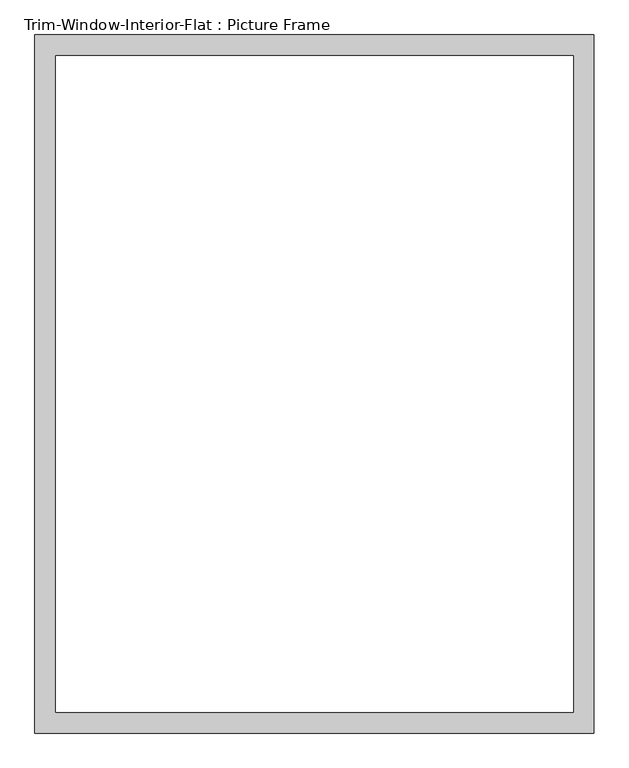
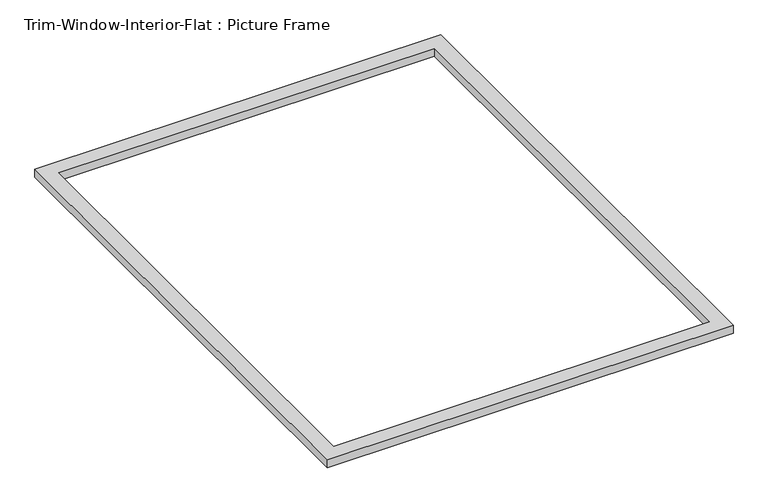
"""IFC4 building model written with IfcOpenShell, lengths in millimetres: proxy geometry, Trim-Window-Interior-Flat : Picture Frame."""

from ifc_helpers import new_model, si_unit, origin, origin_with_axes, place, context, project, spatial, polyline, outline, extrude, source, transform, mapped, element, save


def trim_window_interior_flat_picture_frame_640e2092(model_context):
    return source(origin(), model_context, "Body", "SweptSolid", [
        extrude(outline(polyline([(768.35, -44.45), (-768.35, -44.45), (-768.35, 1873.25), (768.35, 1873.25), (768.35, -44.45)]), holes=[polyline([(711.2, 12.7), (711.2, 1816.1), (-711.2, 1816.1), (-711.2, 12.7), (711.2, 12.7)])]), origin_with_axes(), (0.0, 0.0, 1.0), 31.75),
    ])


if __name__ == "__main__":
    model = new_model("IFC4")
    model_context = context("Model", 3, world=origin())
    ifc_project = project(units=[si_unit("LENGTHUNIT", "METRE", prefix="MILLI")], contexts=[model_context])
    site = spatial("IfcSite", under=ifc_project)
    building = spatial("IfcBuilding", under=site)
    placement = place(None, origin())
    trim_window_interior_flat_picture_frame_shape = trim_window_interior_flat_picture_frame_640e2092(model_context)
    element("IfcBuildingElementProxy", 1, Name="Trim-Window-Interior-Flat : Picture Frame", ObjectType="Trim-Window-Interior-Flat : Picture Frame", at=placement, inside=building, context=model_context, shape_type="MappedRepresentation", body=[
        mapped(trim_window_interior_flat_picture_frame_shape, transform((0.0, 0.0, 0.0), x_axis=(1.0, 0.0, 0.0), y_axis=(0.0, 1.0, 0.0), z_axis=(0.0, 0.0, 1.0))),
    ])
    save(model, "model.ifc")

# Revit data of these elements
# Type "Trim-Window-Interior-Flat : Picture Frame"
#   Trim Thickness_Picture Frame = 0' - 1 1/4"
#   Trim Width = 0' - 2 1/4"
#   Trim Thickness_with Sill = 0' - 0 3/4"
#   Sill Thickness = 0' - 1 1/4"
#   Opening Width [instance default] = 2' - 0"
#   Opening Height [instance default] = 3' - 0"
#   Default Elevation = 4' - 0"
#   Sill = no
#   Picture Frame = yes
#   Trim Material [instance default] = none
# Element 1 (IfcBuildingElementProxy, "Trim-Window-Interior-Flat : Picture Frame")
#   Opening Width = 4' - 9"
#   Opening Height = 6' - 0"
#   Trim Material = Wood - Stained
#   Materials on its faces: "Wood - Stained"
# Materials
#   "Wood - Stained": class "Wood", colour RGB 224 178 126, transparency 0, Cost = 0
